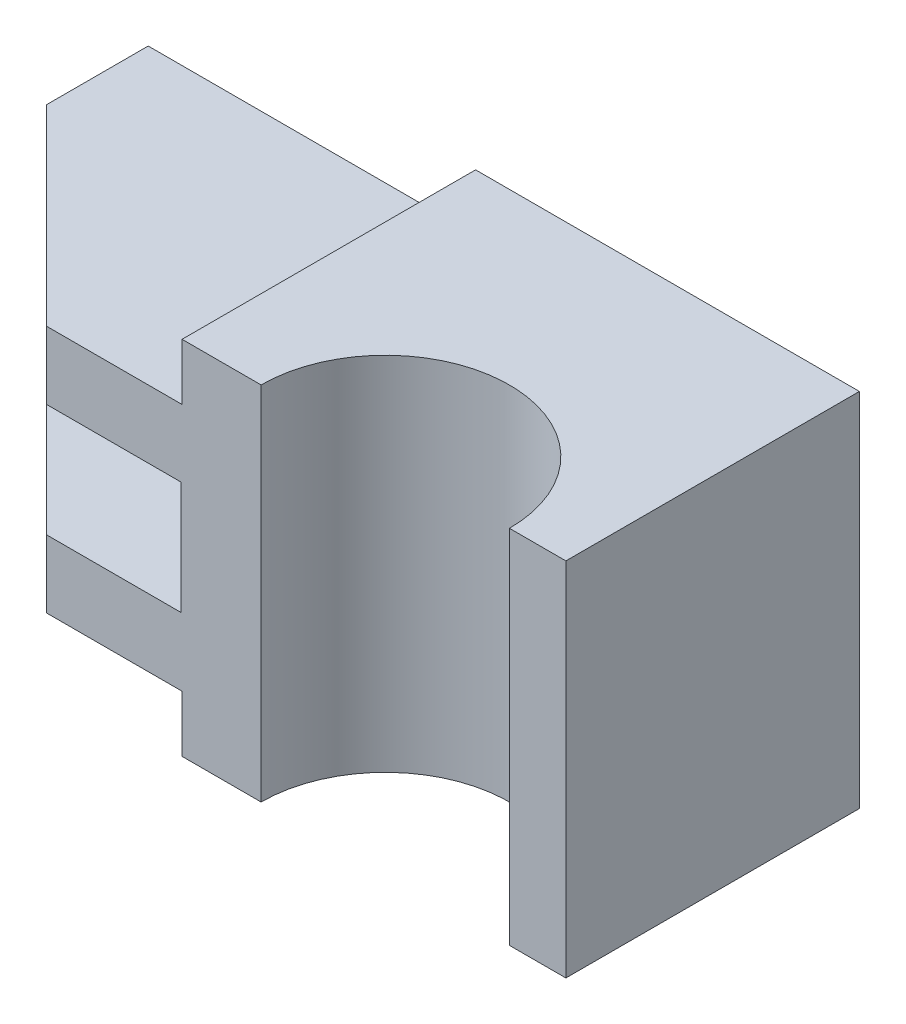
ISO-10303-21;
HEADER;
FILE_DESCRIPTION(('STEP AP214'),'2;1');
FILE_NAME('part.step','',(''),(''),'','','');
FILE_SCHEMA(('AUTOMOTIVE_DESIGN { 1 0 10303 214 1 1 1 1 }'));
ENDSEC;
DATA;
#1=APPLICATION_CONTEXT('core data for automotive mechanical design processes');
#2=APPLICATION_PROTOCOL_DEFINITION('international standard','automotive_design',2000,#1);
#3=PRODUCT_CONTEXT('',#1,'mechanical');
#4=PRODUCT('Part','Part','',(#3));
#5=PRODUCT_RELATED_PRODUCT_CATEGORY('part','',(#4));
#6=PRODUCT_DEFINITION_FORMATION('','',#4);
#7=PRODUCT_DEFINITION_CONTEXT('part definition',#1,'design');
#8=PRODUCT_DEFINITION('design','',#6,#7);
#9=PRODUCT_DEFINITION_SHAPE('','',#8);
#10=(LENGTH_UNIT() NAMED_UNIT(*) SI_UNIT(.MILLI.,.METRE.));
#11=(NAMED_UNIT(*) PLANE_ANGLE_UNIT() SI_UNIT($,.RADIAN.));
#12=(NAMED_UNIT(*) SI_UNIT($,.STERADIAN.) SOLID_ANGLE_UNIT());
#13=UNCERTAINTY_MEASURE_WITH_UNIT(LENGTH_MEASURE(1.E-05),#10,'distance_accuracy_value','');
#14=(GEOMETRIC_REPRESENTATION_CONTEXT(3) GLOBAL_UNCERTAINTY_ASSIGNED_CONTEXT((#13)) GLOBAL_UNIT_ASSIGNED_CONTEXT((#10,
#11,#12)) REPRESENTATION_CONTEXT('',''));
#15=CARTESIAN_POINT('',(0.,0.,0.));
#16=DIRECTION('',(0.,0.,1.));
#17=DIRECTION('',(1.,0.,0.));
#18=AXIS2_PLACEMENT_3D('',#15,#16,#17);
#19=CARTESIAN_POINT('',(-31.5,16.,26.));
#20=DIRECTION('',(1.,0.,0.));
#21=DIRECTION('',(0.,1.,0.));
#22=AXIS2_PLACEMENT_3D('',#19,#20,#21);
#23=PLANE('',#22);
#24=DIRECTION('',(0.,0.,-1.));
#25=VECTOR('',#24,1.);
#26=CARTESIAN_POINT('',(-31.5,-5.00294639462672,26.));
#27=LINE('',#26,#25);
#28=CARTESIAN_POINT('',(-31.5,-5.00294639462672,9.));
#29=VERTEX_POINT('',#28);
#30=CARTESIAN_POINT('',(-31.5,-5.00294639462672,0.));
#31=VERTEX_POINT('',#30);
#32=EDGE_CURVE('E53',#29,#31,#27,.T.);
#33=ORIENTED_EDGE('',*,*,#32,.T.);
#34=DIRECTION('',(0.,-1.,0.));
#35=VECTOR('',#34,1.);
#36=CARTESIAN_POINT('',(-31.5,16.,0.));
#37=LINE('',#36,#35);
#38=CARTESIAN_POINT('',(-31.5,-11.,0.));
#39=VERTEX_POINT('',#38);
#40=EDGE_CURVE('E259',#31,#39,#37,.T.);
#41=ORIENTED_EDGE('',*,*,#40,.T.);
#42=DIRECTION('',(0.,0.,-1.));
#43=VECTOR('',#42,1.);
#44=CARTESIAN_POINT('',(-31.5,-11.,26.));
#45=LINE('',#44,#43);
#46=CARTESIAN_POINT('',(-31.5,-11.,8.99999999999999));
#47=VERTEX_POINT('',#46);
#48=EDGE_CURVE('E211',#47,#39,#45,.T.);
#49=ORIENTED_EDGE('',*,*,#48,.F.);
#50=DIRECTION('',(0.,-1.,0.));
#51=VECTOR('',#50,1.);
#52=CARTESIAN_POINT('',(-31.5,16.,9.));
#53=LINE('',#52,#51);
#54=EDGE_CURVE('E204',#29,#47,#53,.T.);
#55=ORIENTED_EDGE('',*,*,#54,.F.);
#56=EDGE_LOOP('',(#33,#41,#49,#55));
#57=FACE_BOUND('',#56,.T.);
#58=ADVANCED_FACE('F39',(#57),#23,.F.);
#59=CARTESIAN_POINT('',(-20.25,16.,20.25));
#60=DIRECTION('',(0.707106781186548,0.,-0.707106781186548));
#61=DIRECTION('',(-0.707106781186548,0.,-0.707106781186548));
#62=AXIS2_PLACEMENT_3D('',#59,#60,#61);
#63=PLANE('',#62);
#64=DIRECTION('',(0.707106781186548,0.,0.707106781186548));
#65=VECTOR('',#64,1.);
#66=CARTESIAN_POINT('',(-20.25,-5.00294639462672,20.25));
#67=LINE('',#66,#65);
#68=CARTESIAN_POINT('',(-14.5,-5.00294639462672,26.));
#69=VERTEX_POINT('',#68);
#70=EDGE_CURVE('E50',#29,#69,#67,.T.);
#71=ORIENTED_EDGE('',*,*,#70,.F.);
#72=ORIENTED_EDGE('',*,*,#54,.T.);
#73=DIRECTION('',(0.707106781186548,0.,0.707106781186548));
#74=VECTOR('',#73,1.);
#75=CARTESIAN_POINT('',(-20.25,-11.,20.25));
#76=LINE('',#75,#74);
#77=CARTESIAN_POINT('',(-14.5,-11.,26.));
#78=VERTEX_POINT('',#77);
#79=EDGE_CURVE('E269',#47,#78,#76,.T.);
#80=ORIENTED_EDGE('',*,*,#79,.T.);
#81=DIRECTION('',(0.,-1.,0.));
#82=VECTOR('',#81,1.);
#83=CARTESIAN_POINT('',(-14.5,16.,26.));
#84=LINE('',#83,#82);
#85=EDGE_CURVE('E228',#69,#78,#84,.T.);
#86=ORIENTED_EDGE('',*,*,#85,.F.);
#87=EDGE_LOOP('',(#71,#72,#80,#86));
#88=FACE_BOUND('',#87,.T.);
#89=ADVANCED_FACE('F280',(#88),#63,.F.);
#90=CARTESIAN_POINT('',(0.,0.,26.));
#91=DIRECTION('',(0.,0.,1.));
#92=DIRECTION('',(1.,0.,0.));
#93=AXIS2_PLACEMENT_3D('',#90,#91,#92);
#94=PLANE('',#93);
#95=DIRECTION('',(1.,0.,0.));
#96=VECTOR('',#95,1.);
#97=CARTESIAN_POINT('',(0.,5.,26.));
#98=LINE('',#97,#96);
#99=CARTESIAN_POINT('',(-14.5,5.,26.));
#100=VERTEX_POINT('',#99);
#101=CARTESIAN_POINT('',(-2.59243585903388,5.,26.));
#102=VERTEX_POINT('',#101);
#103=EDGE_CURVE('E154',#100,#102,#98,.T.);
#104=ORIENTED_EDGE('',*,*,#103,.T.);
#105=DIRECTION('',(0.,-1.,0.));
#106=VECTOR('',#105,1.);
#107=CARTESIAN_POINT('',(-2.59243585903388,0.,26.));
#108=LINE('',#107,#106);
#109=CARTESIAN_POINT('',(-2.59243585903388,-5.00294639462672,26.));
#110=VERTEX_POINT('',#109);
#111=EDGE_CURVE('E168',#102,#110,#108,.T.);
#112=ORIENTED_EDGE('',*,*,#111,.T.);
#113=DIRECTION('',(1.,0.,0.));
#114=VECTOR('',#113,1.);
#115=CARTESIAN_POINT('',(0.,-5.00294639462672,26.));
#116=LINE('',#115,#114);
#117=EDGE_CURVE('E162',#69,#110,#116,.T.);
#118=ORIENTED_EDGE('',*,*,#117,.F.);
#119=ORIENTED_EDGE('',*,*,#85,.T.);
#120=DIRECTION('',(1.,0.,0.));
#121=VECTOR('',#120,1.);
#122=CARTESIAN_POINT('',(-31.5,-11.,26.));
#123=LINE('',#122,#121);
#124=CARTESIAN_POINT('',(-2.50000000000001,-11.,26.));
#125=VERTEX_POINT('',#124);
#126=EDGE_CURVE('E210',#78,#125,#123,.T.);
#127=ORIENTED_EDGE('',*,*,#126,.T.);
#128=DIRECTION('',(0.,-1.,0.));
#129=VECTOR('',#128,1.);
#130=CARTESIAN_POINT('',(-2.50000000000001,-16.,26.));
#131=LINE('',#130,#129);
#132=CARTESIAN_POINT('',(-2.50000000000001,-16.,26.));
#133=VERTEX_POINT('',#132);
#134=EDGE_CURVE('E208',#125,#133,#131,.T.);
#135=ORIENTED_EDGE('',*,*,#134,.T.);
#136=DIRECTION('',(1.,0.,0.));
#137=VECTOR('',#136,1.);
#138=CARTESIAN_POINT('',(-31.5,-16.,26.));
#139=LINE('',#138,#137);
#140=CARTESIAN_POINT('',(4.5,-16.,26.));
#141=VERTEX_POINT('',#140);
#142=EDGE_CURVE('E249',#133,#141,#139,.T.);
#143=ORIENTED_EDGE('',*,*,#142,.T.);
#144=DIRECTION('',(0.,-1.,0.));
#145=VECTOR('',#144,1.);
#146=CARTESIAN_POINT('',(4.5,16.,26.));
#147=LINE('',#146,#145);
#148=CARTESIAN_POINT('',(4.5,16.,26.));
#149=VERTEX_POINT('',#148);
#150=EDGE_CURVE('E231',#149,#141,#147,.T.);
#151=ORIENTED_EDGE('',*,*,#150,.F.);
#152=DIRECTION('',(-1.,0.,0.));
#153=VECTOR('',#152,1.);
#154=CARTESIAN_POINT('',(-31.5,16.,26.));
#155=LINE('',#154,#153);
#156=CARTESIAN_POINT('',(-2.50000000000001,16.,26.));
#157=VERTEX_POINT('',#156);
#158=EDGE_CURVE('E242',#149,#157,#155,.T.);
#159=ORIENTED_EDGE('',*,*,#158,.T.);
#160=DIRECTION('',(0.,-1.,0.));
#161=VECTOR('',#160,1.);
#162=CARTESIAN_POINT('',(-2.50000000000001,16.,26.));
#163=LINE('',#162,#161);
#164=CARTESIAN_POINT('',(-2.50000000000001,11.,26.));
#165=VERTEX_POINT('',#164);
#166=EDGE_CURVE('E188',#157,#165,#163,.T.);
#167=ORIENTED_EDGE('',*,*,#166,.T.);
#168=DIRECTION('',(-1.,0.,0.));
#169=VECTOR('',#168,1.);
#170=CARTESIAN_POINT('',(-31.5,11.,26.));
#171=LINE('',#170,#169);
#172=CARTESIAN_POINT('',(-14.5,11.,26.));
#173=VERTEX_POINT('',#172);
#174=EDGE_CURVE('E194',#165,#173,#171,.T.);
#175=ORIENTED_EDGE('',*,*,#174,.T.);
#176=EDGE_CURVE('E174',#173,#100,#84,.T.);
#177=ORIENTED_EDGE('',*,*,#176,.T.);
#178=EDGE_LOOP('',(#104,#112,#118,#119,#127,#135,#143,#151,#159,#167,#175,#177));
#179=FACE_BOUND('',#178,.T.);
#180=ADVANCED_FACE('F175',(#179),#94,.T.);
#181=CARTESIAN_POINT('',(31.5,16.,26.));
#182=DIRECTION('',(-1.,0.,0.));
#183=DIRECTION('',(0.,-1.,0.));
#184=AXIS2_PLACEMENT_3D('',#181,#182,#183);
#185=PLANE('',#184);
#186=DIRECTION('',(0.,1.,0.));
#187=VECTOR('',#186,1.);
#188=CARTESIAN_POINT('',(31.5,16.,0.));
#189=LINE('',#188,#187);
#190=CARTESIAN_POINT('',(31.5,-16.,0.));
#191=VERTEX_POINT('',#190);
#192=CARTESIAN_POINT('',(31.5,16.,0.));
#193=VERTEX_POINT('',#192);
#194=EDGE_CURVE('E238',#191,#193,#189,.T.);
#195=ORIENTED_EDGE('',*,*,#194,.T.);
#196=DIRECTION('',(0.,0.,-1.));
#197=VECTOR('',#196,1.);
#198=CARTESIAN_POINT('',(31.5,16.,26.));
#199=LINE('',#198,#197);
#200=CARTESIAN_POINT('',(31.5,16.,26.));
#201=VERTEX_POINT('',#200);
#202=EDGE_CURVE('E264',#201,#193,#199,.T.);
#203=ORIENTED_EDGE('',*,*,#202,.F.);
#204=DIRECTION('',(0.,1.,0.));
#205=VECTOR('',#204,1.);
#206=CARTESIAN_POINT('',(31.5,16.,26.));
#207=LINE('',#206,#205);
#208=CARTESIAN_POINT('',(31.5,-16.,26.));
#209=VERTEX_POINT('',#208);
#210=EDGE_CURVE('E241',#209,#201,#207,.T.);
#211=ORIENTED_EDGE('',*,*,#210,.F.);
#212=DIRECTION('',(0.,0.,-1.));
#213=VECTOR('',#212,1.);
#214=CARTESIAN_POINT('',(31.5,-16.,26.));
#215=LINE('',#214,#213);
#216=EDGE_CURVE('E255',#209,#191,#215,.T.);
#217=ORIENTED_EDGE('',*,*,#216,.T.);
#218=EDGE_LOOP('',(#195,#203,#211,#217));
#219=FACE_BOUND('',#218,.T.);
#220=ADVANCED_FACE('F41',(#219),#185,.F.);
#221=CARTESIAN_POINT('',(-31.5,16.,26.));
#222=DIRECTION('',(0.,-1.,0.));
#223=DIRECTION('',(0.,0.,-1.));
#224=AXIS2_PLACEMENT_3D('',#221,#222,#223);
#225=PLANE('',#224);
#226=DIRECTION('',(-1.,0.,0.));
#227=VECTOR('',#226,1.);
#228=CARTESIAN_POINT('',(-31.5,16.,0.));
#229=LINE('',#228,#227);
#230=CARTESIAN_POINT('',(-2.50000000000001,16.,0.));
#231=VERTEX_POINT('',#230);
#232=EDGE_CURVE('E253',#193,#231,#229,.T.);
#233=ORIENTED_EDGE('',*,*,#232,.T.);
#234=DIRECTION('',(0.,0.,-1.));
#235=VECTOR('',#234,1.);
#236=CARTESIAN_POINT('',(-2.50000000000001,16.,26.));
#237=LINE('',#236,#235);
#238=EDGE_CURVE('E196',#157,#231,#237,.T.);
#239=ORIENTED_EDGE('',*,*,#238,.F.);
#240=ORIENTED_EDGE('',*,*,#158,.F.);
#241=CARTESIAN_POINT('',(15.5,16.,26.));
#242=DIRECTION('',(0.,-1.,0.));
#243=DIRECTION('',(0.,0.,-1.));
#244=AXIS2_PLACEMENT_3D('',#241,#242,#243);
#245=CIRCLE('',#244,11.);
#246=CARTESIAN_POINT('',(26.5,16.,26.));
#247=VERTEX_POINT('',#246);
#248=EDGE_CURVE('E229',#149,#247,#245,.T.);
#249=ORIENTED_EDGE('',*,*,#248,.T.);
#250=EDGE_CURVE('E246',#201,#247,#155,.T.);
#251=ORIENTED_EDGE('',*,*,#250,.F.);
#252=ORIENTED_EDGE('',*,*,#202,.T.);
#253=EDGE_LOOP('',(#233,#239,#240,#249,#251,#252));
#254=FACE_BOUND('',#253,.T.);
#255=ADVANCED_FACE('F306',(#254),#225,.F.);
#256=CARTESIAN_POINT('',(-31.5,11.,0.));
#257=VERTEX_POINT('',#256);
#258=CARTESIAN_POINT('',(-31.5,5.,0.));
#259=VERTEX_POINT('',#258);
#260=EDGE_CURVE('E256',#257,#259,#37,.T.);
#261=ORIENTED_EDGE('',*,*,#260,.T.);
#262=DIRECTION('',(0.,0.,-1.));
#263=VECTOR('',#262,1.);
#264=CARTESIAN_POINT('',(-31.5,5.,26.));
#265=LINE('',#264,#263);
#266=CARTESIAN_POINT('',(-31.5,5.,9.));
#267=VERTEX_POINT('',#266);
#268=EDGE_CURVE('E184',#267,#259,#265,.T.);
#269=ORIENTED_EDGE('',*,*,#268,.F.);
#270=CARTESIAN_POINT('',(-31.5,11.,9.));
#271=VERTEX_POINT('',#270);
#272=EDGE_CURVE('E227',#271,#267,#53,.T.);
#273=ORIENTED_EDGE('',*,*,#272,.F.);
#274=DIRECTION('',(0.,0.,-1.));
#275=VECTOR('',#274,1.);
#276=CARTESIAN_POINT('',(-31.5,11.,26.));
#277=LINE('',#276,#275);
#278=EDGE_CURVE('E65',#271,#257,#277,.T.);
#279=ORIENTED_EDGE('',*,*,#278,.T.);
#280=EDGE_LOOP('',(#261,#269,#273,#279));
#281=FACE_BOUND('',#280,.T.);
#282=ADVANCED_FACE('F318',(#281),#23,.F.);
#283=CARTESIAN_POINT('',(-31.5,-16.,26.));
#284=DIRECTION('',(0.,1.,0.));
#285=DIRECTION('',(0.,0.,1.));
#286=AXIS2_PLACEMENT_3D('',#283,#284,#285);
#287=PLANE('',#286);
#288=ORIENTED_EDGE('',*,*,#142,.F.);
#289=DIRECTION('',(0.,0.,-1.));
#290=VECTOR('',#289,1.);
#291=CARTESIAN_POINT('',(-2.50000000000001,-16.,26.));
#292=LINE('',#291,#290);
#293=CARTESIAN_POINT('',(-2.50000000000001,-16.,0.));
#294=VERTEX_POINT('',#293);
#295=EDGE_CURVE('E199',#133,#294,#292,.T.);
#296=ORIENTED_EDGE('',*,*,#295,.T.);
#297=DIRECTION('',(1.,0.,0.));
#298=VECTOR('',#297,1.);
#299=CARTESIAN_POINT('',(-31.5,-16.,0.));
#300=LINE('',#299,#298);
#301=EDGE_CURVE('E244',#294,#191,#300,.T.);
#302=ORIENTED_EDGE('',*,*,#301,.T.);
#303=ORIENTED_EDGE('',*,*,#216,.F.);
#304=CARTESIAN_POINT('',(26.5,-16.,26.));
#305=VERTEX_POINT('',#304);
#306=EDGE_CURVE('E248',#305,#209,#139,.T.);
#307=ORIENTED_EDGE('',*,*,#306,.F.);
#308=CARTESIAN_POINT('',(15.5,-16.,26.));
#309=DIRECTION('',(0.,-1.,0.));
#310=DIRECTION('',(0.,0.,-1.));
#311=AXIS2_PLACEMENT_3D('',#308,#309,#310);
#312=CIRCLE('',#311,11.);
#313=EDGE_CURVE('E223',#141,#305,#312,.T.);
#314=ORIENTED_EDGE('',*,*,#313,.F.);
#315=EDGE_LOOP('',(#288,#296,#302,#303,#307,#314));
#316=FACE_BOUND('',#315,.T.);
#317=ADVANCED_FACE('F298',(#316),#287,.F.);
#318=DIRECTION('',(0.,-1.,0.));
#319=VECTOR('',#318,1.);
#320=CARTESIAN_POINT('',(26.5,16.,26.));
#321=LINE('',#320,#319);
#322=EDGE_CURVE('E232',#247,#305,#321,.T.);
#323=ORIENTED_EDGE('',*,*,#322,.T.);
#324=ORIENTED_EDGE('',*,*,#306,.T.);
#325=ORIENTED_EDGE('',*,*,#210,.T.);
#326=ORIENTED_EDGE('',*,*,#250,.T.);
#327=EDGE_LOOP('',(#323,#324,#325,#326));
#328=FACE_BOUND('',#327,.T.);
#329=ADVANCED_FACE('F305',(#328),#94,.T.);
#330=CARTESIAN_POINT('',(0.,0.,0.));
#331=DIRECTION('',(0.,0.,1.));
#332=DIRECTION('',(1.,0.,0.));
#333=AXIS2_PLACEMENT_3D('',#330,#331,#332);
#334=PLANE('',#333);
#335=DIRECTION('',(0.,-1.,0.));
#336=VECTOR('',#335,1.);
#337=CARTESIAN_POINT('',(-2.59243585903388,0.,0.));
#338=LINE('',#337,#336);
#339=CARTESIAN_POINT('',(-2.59243585903388,5.,0.));
#340=VERTEX_POINT('',#339);
#341=CARTESIAN_POINT('',(-2.59243585903388,-5.00294639462672,0.));
#342=VERTEX_POINT('',#341);
#343=EDGE_CURVE('E177',#340,#342,#338,.T.);
#344=ORIENTED_EDGE('',*,*,#343,.F.);
#345=DIRECTION('',(1.,0.,0.));
#346=VECTOR('',#345,1.);
#347=CARTESIAN_POINT('',(0.,5.,0.));
#348=LINE('',#347,#346);
#349=EDGE_CURVE('E160',#259,#340,#348,.T.);
#350=ORIENTED_EDGE('',*,*,#349,.F.);
#351=ORIENTED_EDGE('',*,*,#260,.F.);
#352=DIRECTION('',(-1.,0.,0.));
#353=VECTOR('',#352,1.);
#354=CARTESIAN_POINT('',(-31.5,11.,0.));
#355=LINE('',#354,#353);
#356=CARTESIAN_POINT('',(-2.50000000000001,11.,0.));
#357=VERTEX_POINT('',#356);
#358=EDGE_CURVE('E191',#357,#257,#355,.T.);
#359=ORIENTED_EDGE('',*,*,#358,.F.);
#360=DIRECTION('',(0.,-1.,0.));
#361=VECTOR('',#360,1.);
#362=CARTESIAN_POINT('',(-2.50000000000001,16.,0.));
#363=LINE('',#362,#361);
#364=EDGE_CURVE('E200',#231,#357,#363,.T.);
#365=ORIENTED_EDGE('',*,*,#364,.F.);
#366=ORIENTED_EDGE('',*,*,#232,.F.);
#367=ORIENTED_EDGE('',*,*,#194,.F.);
#368=ORIENTED_EDGE('',*,*,#301,.F.);
#369=DIRECTION('',(0.,-1.,0.));
#370=VECTOR('',#369,1.);
#371=CARTESIAN_POINT('',(-2.50000000000001,-16.,0.));
#372=LINE('',#371,#370);
#373=CARTESIAN_POINT('',(-2.50000000000001,-11.,0.));
#374=VERTEX_POINT('',#373);
#375=EDGE_CURVE('E212',#374,#294,#372,.T.);
#376=ORIENTED_EDGE('',*,*,#375,.F.);
#377=DIRECTION('',(1.,0.,0.));
#378=VECTOR('',#377,1.);
#379=CARTESIAN_POINT('',(-31.5,-11.,0.));
#380=LINE('',#379,#378);
#381=EDGE_CURVE('E190',#39,#374,#380,.T.);
#382=ORIENTED_EDGE('',*,*,#381,.F.);
#383=ORIENTED_EDGE('',*,*,#40,.F.);
#384=DIRECTION('',(1.,0.,0.));
#385=VECTOR('',#384,1.);
#386=CARTESIAN_POINT('',(0.,-5.00294639462672,0.));
#387=LINE('',#386,#385);
#388=EDGE_CURVE('E176',#31,#342,#387,.T.);
#389=ORIENTED_EDGE('',*,*,#388,.T.);
#390=EDGE_LOOP('',(#344,#350,#351,#359,#365,#366,#367,#368,#376,#382,#383,#389));
#391=FACE_BOUND('',#390,.T.);
#392=ADVANCED_FACE('F287',(#391),#334,.F.);
#393=CARTESIAN_POINT('',(15.5,16.,26.));
#394=DIRECTION('',(0.,-1.,0.));
#395=DIRECTION('',(0.,0.,-1.));
#396=AXIS2_PLACEMENT_3D('',#393,#394,#395);
#397=CYLINDRICAL_SURFACE('',#396,11.);
#398=ORIENTED_EDGE('',*,*,#313,.T.);
#399=ORIENTED_EDGE('',*,*,#322,.F.);
#400=ORIENTED_EDGE('',*,*,#248,.F.);
#401=ORIENTED_EDGE('',*,*,#150,.T.);
#402=EDGE_LOOP('',(#398,#399,#400,#401));
#403=FACE_BOUND('',#402,.T.);
#404=ADVANCED_FACE('F297',(#403),#397,.F.);
#405=ORIENTED_EDGE('',*,*,#272,.T.);
#406=DIRECTION('',(0.707106781186548,0.,0.707106781186548));
#407=VECTOR('',#406,1.);
#408=CARTESIAN_POINT('',(-20.25,5.,20.25));
#409=LINE('',#408,#407);
#410=EDGE_CURVE('E11',#267,#100,#409,.T.);
#411=ORIENTED_EDGE('',*,*,#410,.T.);
#412=ORIENTED_EDGE('',*,*,#176,.F.);
#413=DIRECTION('',(-0.707106781186548,0.,-0.707106781186548));
#414=VECTOR('',#413,1.);
#415=CARTESIAN_POINT('',(-20.25,11.,20.25));
#416=LINE('',#415,#414);
#417=EDGE_CURVE('E272',#173,#271,#416,.T.);
#418=ORIENTED_EDGE('',*,*,#417,.T.);
#419=EDGE_LOOP('',(#405,#411,#412,#418));
#420=FACE_BOUND('',#419,.T.);
#421=ADVANCED_FACE('F324',(#420),#63,.F.);
#422=CARTESIAN_POINT('',(-31.5,-11.,26.));
#423=DIRECTION('',(0.,1.,0.));
#424=DIRECTION('',(-1.,0.,0.));
#425=AXIS2_PLACEMENT_3D('',#422,#423,#424);
#426=PLANE('',#425);
#427=ORIENTED_EDGE('',*,*,#48,.T.);
#428=ORIENTED_EDGE('',*,*,#381,.T.);
#429=DIRECTION('',(0.,0.,-1.));
#430=VECTOR('',#429,1.);
#431=CARTESIAN_POINT('',(-2.50000000000001,-11.,26.));
#432=LINE('',#431,#430);
#433=EDGE_CURVE('E219',#125,#374,#432,.T.);
#434=ORIENTED_EDGE('',*,*,#433,.F.);
#435=ORIENTED_EDGE('',*,*,#126,.F.);
#436=ORIENTED_EDGE('',*,*,#79,.F.);
#437=EDGE_LOOP('',(#427,#428,#434,#435,#436));
#438=FACE_BOUND('',#437,.T.);
#439=ADVANCED_FACE('F281',(#438),#426,.F.);
#440=CARTESIAN_POINT('',(-2.50000000000001,-16.,26.));
#441=DIRECTION('',(1.,0.,0.));
#442=DIRECTION('',(0.,0.,-1.));
#443=AXIS2_PLACEMENT_3D('',#440,#441,#442);
#444=PLANE('',#443);
#445=ORIENTED_EDGE('',*,*,#375,.T.);
#446=ORIENTED_EDGE('',*,*,#295,.F.);
#447=ORIENTED_EDGE('',*,*,#134,.F.);
#448=ORIENTED_EDGE('',*,*,#433,.T.);
#449=EDGE_LOOP('',(#445,#446,#447,#448));
#450=FACE_BOUND('',#449,.T.);
#451=ADVANCED_FACE('F293',(#450),#444,.F.);
#452=CARTESIAN_POINT('',(-31.5,11.,26.));
#453=DIRECTION('',(0.,-1.,0.));
#454=DIRECTION('',(1.,0.,0.));
#455=AXIS2_PLACEMENT_3D('',#452,#453,#454);
#456=PLANE('',#455);
#457=ORIENTED_EDGE('',*,*,#174,.F.);
#458=DIRECTION('',(0.,0.,-1.));
#459=VECTOR('',#458,1.);
#460=CARTESIAN_POINT('',(-2.50000000000001,11.,26.));
#461=LINE('',#460,#459);
#462=EDGE_CURVE('E201',#165,#357,#461,.T.);
#463=ORIENTED_EDGE('',*,*,#462,.T.);
#464=ORIENTED_EDGE('',*,*,#358,.T.);
#465=ORIENTED_EDGE('',*,*,#278,.F.);
#466=ORIENTED_EDGE('',*,*,#417,.F.);
#467=EDGE_LOOP('',(#457,#463,#464,#465,#466));
#468=FACE_BOUND('',#467,.T.);
#469=ADVANCED_FACE('F320',(#468),#456,.F.);
#470=CARTESIAN_POINT('',(-2.50000000000001,16.,26.));
#471=DIRECTION('',(1.,0.,0.));
#472=DIRECTION('',(0.,0.,-1.));
#473=AXIS2_PLACEMENT_3D('',#470,#471,#472);
#474=PLANE('',#473);
#475=ORIENTED_EDGE('',*,*,#364,.T.);
#476=ORIENTED_EDGE('',*,*,#462,.F.);
#477=ORIENTED_EDGE('',*,*,#166,.F.);
#478=ORIENTED_EDGE('',*,*,#238,.T.);
#479=EDGE_LOOP('',(#475,#476,#477,#478));
#480=FACE_BOUND('',#479,.T.);
#481=ADVANCED_FACE('F315',(#480),#474,.F.);
#482=CARTESIAN_POINT('',(0.,5.,26.));
#483=DIRECTION('',(0.,1.,0.));
#484=DIRECTION('',(0.,0.,1.));
#485=AXIS2_PLACEMENT_3D('',#482,#483,#484);
#486=PLANE('',#485);
#487=ORIENTED_EDGE('',*,*,#268,.T.);
#488=ORIENTED_EDGE('',*,*,#349,.T.);
#489=DIRECTION('',(0.,0.,-1.));
#490=VECTOR('',#489,1.);
#491=CARTESIAN_POINT('',(-2.59243585903388,5.,26.));
#492=LINE('',#491,#490);
#493=EDGE_CURVE('E151',#102,#340,#492,.T.);
#494=ORIENTED_EDGE('',*,*,#493,.F.);
#495=ORIENTED_EDGE('',*,*,#103,.F.);
#496=ORIENTED_EDGE('',*,*,#410,.F.);
#497=EDGE_LOOP('',(#487,#488,#494,#495,#496));
#498=FACE_BOUND('',#497,.T.);
#499=ADVANCED_FACE('F153',(#498),#486,.F.);
#500=CARTESIAN_POINT('',(0.,-5.00294639462672,26.));
#501=DIRECTION('',(0.,1.,0.));
#502=DIRECTION('',(0.,0.,1.));
#503=AXIS2_PLACEMENT_3D('',#500,#501,#502);
#504=PLANE('',#503);
#505=ORIENTED_EDGE('',*,*,#70,.T.);
#506=ORIENTED_EDGE('',*,*,#117,.T.);
#507=DIRECTION('',(0.,0.,-1.));
#508=VECTOR('',#507,1.);
#509=CARTESIAN_POINT('',(-2.59243585903388,-5.00294639462672,26.));
#510=LINE('',#509,#508);
#511=EDGE_CURVE('E163',#110,#342,#510,.T.);
#512=ORIENTED_EDGE('',*,*,#511,.T.);
#513=ORIENTED_EDGE('',*,*,#388,.F.);
#514=ORIENTED_EDGE('',*,*,#32,.F.);
#515=EDGE_LOOP('',(#505,#506,#512,#513,#514));
#516=FACE_BOUND('',#515,.T.);
#517=ADVANCED_FACE('F275',(#516),#504,.T.);
#518=CARTESIAN_POINT('',(-2.59243585903388,0.,26.));
#519=DIRECTION('',(1.,0.,0.));
#520=DIRECTION('',(0.,0.,-1.));
#521=AXIS2_PLACEMENT_3D('',#518,#519,#520);
#522=PLANE('',#521);
#523=ORIENTED_EDGE('',*,*,#343,.T.);
#524=ORIENTED_EDGE('',*,*,#511,.F.);
#525=ORIENTED_EDGE('',*,*,#111,.F.);
#526=ORIENTED_EDGE('',*,*,#493,.T.);
#527=EDGE_LOOP('',(#523,#524,#525,#526));
#528=FACE_BOUND('',#527,.T.);
#529=ADVANCED_FACE('F170',(#528),#522,.F.);
#530=CLOSED_SHELL('',(#58,#89,#180,#220,#255,#282,#317,#329,#392,#404,#421,#439,#451,#469,#481,
#499,#517,#529));
#531=MANIFOLD_SOLID_BREP('B2',#530);
#532=ADVANCED_BREP_SHAPE_REPRESENTATION('',(#18,#531),#14);
#533=SHAPE_DEFINITION_REPRESENTATION(#9,#532);
ENDSEC;
END-ISO-10303-21;
